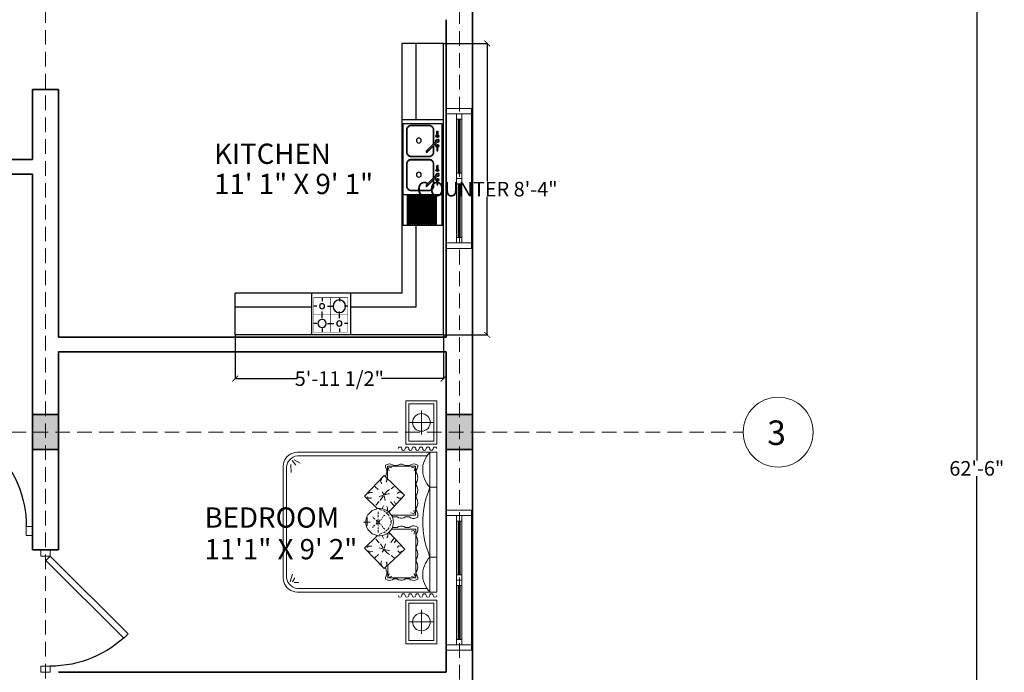
# Model space of a CAD drawing. Units: inches. Extents: x 782 to 2660, y -1008 to 166.
# Tile 6 of 12: x 1251 to 1589, y -400 to -176. Entities that reach past the tile are written whole.
import ezdxf

# ---------------------------------------------------------------- set-up
doc = ezdxf.new("R2010")
doc.units = ezdxf.units.IN
doc.header["$MEASUREMENT"] = 0
doc.linetypes.add('DASHED', pattern=[0.75, 0.5, -0.25])
for name, color, linetype, lineweight in [('A-ANNO-DIMS', 4, 'Continuous', 18), ('A-AREA-IDEN', 4, 'Continuous', 18), ('A-COLS', 7, 'Continuous', 35), ('A-Door', 150, 'Continuous', 18), ('A-FLOR-FIXT', 9, 'Continuous', 18), ('A-FURN', 8, 'Continuous', 13), ('A-Glaz', 4, 'Continuous', 18), ('A-GRID', 8, 'DASHED', 13), ('A-GRID-IDEN', 7, 'Continuous', 18), ('A-WALL', 7, 'Continuous', 35)]:
    doc.layers.add(name, color=color, linetype=linetype, lineweight=lineweight)
doc.layers.add('NET 01', color=8, linetype='Continuous')
doc.layers.add('TEFRIS', color=11, linetype='Continuous')
doc.styles.get("Standard").update_dxf_attribs({"font": 'arial.ttf'})
doc.dimstyles.get("Standard").update_dxf_attribs({"dimtxt": 5, "dimasz": 2, "dimexe": 0.18, "dimexo": 0.0625, "dimgap": 0.09, "dimtad": 0, "dimtih": 1, "dimtoh": 1, "dimdec": 0, "dimzin": 0, "dimdsep": 46, "dimlunit": 3, "dimtxsty": 'Standard', "dimblk": 'ARCHTICK', "dimcen": 0.09, "dimadec": 0, "dimazin": 0, "dimtfac": 1, "dimtdec": 0, "dimtofl": 0, "dimtmove": 0, "dimatfit": 3, "dimfxl": 1, "dimtolj": 1, "dimtzin": 0, "dimarcsym": 0})

# ---------------------------------------------------------------- blocks, each defined once
blk = doc.blocks.new('A$C592222DF')
at = {"layer": 'A-Door'}
for points in [[(-0.0354, -0.0354), (-0.6718, 0.601), (-0.6364, 0.6364), (0, 0)], [(-0.95, 0), (-0.95, -0.075), (-0.9, -0.075), (-0.9, 0)], [(0, 0), (0, -0.075), (0.05, -0.075), (0.05, 0)]]:
    blk.add_lwpolyline(points, close=True, dxfattribs=at)
at = {"layer": 'NET 01'}
blk.add_arc((0, 0), 0.9, 135, 180, dxfattribs=at)
blk = doc.blocks.new('d-bed-4')
at = {"color": 0, "linetype": 'ByBlock'}
for p, q in [((0.56, 0), (0, 0)), ((0, 0), (0, -0.4)), ((0.56, -0.4), (0.56, 0)), ((0.664, -1.8), (0.664, 0)), ((0.664, 0), (2.464, 0)), ((0.664, 0), (2.464, 0)), ((0.664, -1.8), (0.664, 0)), ((1.114, 0), (1.114, -0.09)), ((2.014, 0), (2.014, -0.09)), ((2.464, 0), (2.464, -1.8)), ((2.464, 0), (2.464, -1.8)), ((2.568, -0.4), (2.568, 0)), ((2.568, 0), (3.128, 0)), ((3.128, 0), (3.128, -0.4)), ((0.52, -0.04), (0.04, -0.04)), ((0.04, -0.04), (0.04, -0.36)), ((0.28, -0.046), (0.28, -0.354)), ((0.52, -0.36), (0.52, -0.04)), ((2.464, -0.09), (0.664, -0.09)), ((0.664, -0.09), (0.689, -0.112)), ((0.689, -0.112), (0.716, -0.131)), ((1.064, -0.131), (1.091, -0.112)), ((1.091, -0.112), (1.114, -0.09)), ((1.114, -0.09), (1.181, -0.115)), ((1.181, -0.115), (1.249, -0.137)), ((1.879, -0.137), (1.947, -0.115)), ((1.947, -0.115), (2.014, -0.09)), ((2.014, -0.09), (2.037, -0.112)), ((2.037, -0.112), (2.064, -0.131)), ((2.412, -0.131), (2.439, -0.112)), ((2.439, -0.112), (2.464, -0.09)), ((2.608, -0.36), (2.608, -0.04)), ((2.608, -0.04), (3.088, -0.04)), ((2.848, -0.046), (2.848, -0.354)), ((3.088, -0.04), (3.088, -0.36)), ((0.126, -0.2), (0.434, -0.2)), ((0.709, -1.795), (0.709, -0.128)), ((0.716, -0.131), (0.745, -0.148)), ((0.745, -0.148), (0.776, -0.162)), ((0.776, -0.162), (0.806, -0.173)), ((0.806, -0.173), (0.84, -0.18)), ((0.821, -0.268), (0.831, -0.248)), ((0.831, -0.248), (0.853, -0.248)), ((0.84, -0.18), (0.873, -0.184)), ((0.853, -0.248), (0.875, -0.256)), ((0.873, -0.184), (0.907, -0.184)), ((0.907, -0.184), (0.939, -0.18)), ((0.939, -0.18), (0.972, -0.173)), ((0.947, -0.256), (0.968, -0.25)), ((0.968, -0.25), (0.99, -0.248)), ((0.972, -0.173), (1.004, -0.162)), ((0.99, -0.248), (1.013, -0.25)), ((1.004, -0.162), (1.035, -0.148)), ((1.013, -0.25), (1.035, -0.256)), ((1.035, -0.148), (1.064, -0.131)), ((1.109, -0.256), (1.13, -0.25)), ((1.13, -0.25), (1.152, -0.248)), ((1.152, -0.248), (1.175, -0.25)), ((1.175, -0.25), (1.197, -0.256)), ((1.249, -0.137), (1.317, -0.155)), ((1.269, -0.256), (1.29, -0.25)), ((1.29, -0.25), (1.314, -0.248)), ((1.314, -0.248), (1.337, -0.25)), ((1.317, -0.155), (1.388, -0.169)), ((1.337, -0.25), (1.359, -0.256)), ((1.388, -0.169), (1.458, -0.178)), ((1.431, -0.256), (1.451, -0.248)), ((1.451, -0.248), (1.474, -0.248)), ((1.458, -0.178), (1.528, -0.182)), ((1.474, -0.248), (1.501, -0.248)), ((1.501, -0.248), (1.51, -0.268)), ((1.528, -0.182), (1.6, -0.182)), ((1.6, -0.182), (1.67, -0.178)), ((1.627, -0.248), (1.618, -0.268)), ((1.654, -0.248), (1.627, -0.248)), ((1.677, -0.248), (1.654, -0.248)), ((1.67, -0.178), (1.74, -0.169)), ((1.697, -0.256), (1.677, -0.248)), ((1.74, -0.169), (1.811, -0.155)), ((1.791, -0.25), (1.769, -0.256)), ((1.814, -0.248), (1.791, -0.25)), ((1.811, -0.155), (1.879, -0.137)), ((1.838, -0.25), (1.814, -0.248)), ((1.859, -0.256), (1.838, -0.25)), ((1.953, -0.25), (1.931, -0.256)), ((1.976, -0.248), (1.953, -0.25)), ((1.998, -0.25), (1.976, -0.248)), ((2.019, -0.256), (1.998, -0.25)), ((2.064, -0.131), (2.093, -0.148)), ((2.093, -0.148), (2.124, -0.162)), ((2.115, -0.25), (2.093, -0.256)), ((2.138, -0.248), (2.115, -0.25)), ((2.124, -0.162), (2.156, -0.173)), ((2.16, -0.25), (2.138, -0.248)), ((2.156, -0.173), (2.189, -0.18)), ((2.181, -0.256), (2.16, -0.25)), ((2.189, -0.18), (2.221, -0.184)), ((2.221, -0.184), (2.255, -0.184)), ((2.275, -0.248), (2.253, -0.256)), ((2.255, -0.184), (2.288, -0.18)), ((2.297, -0.248), (2.275, -0.248)), ((2.288, -0.18), (2.322, -0.173)), ((2.307, -0.268), (2.297, -0.248)), ((2.322, -0.173), (2.352, -0.162)), ((2.352, -0.162), (2.383, -0.148)), ((2.383, -0.148), (2.412, -0.131)), ((2.419, -0.128), (2.419, -1.795)), ((3.002, -0.2), (2.694, -0.2)), ((0.04, -0.36), (0.52, -0.36)), ((0.815, -0.292), (0.821, -0.268)), ((0.817, -0.315), (0.815, -0.292)), ((0.824, -0.337), (0.817, -0.315)), ((0.835, -0.356), (0.824, -0.337)), ((0.835, -0.405), (0.835, -0.356)), ((0.844, -0.635), (0.844, -0.275)), ((0.844, -0.275), (1.472, -0.275)), ((0.857, -0.293), (0.866, -0.329)), ((0.862, -0.281), (0.902, -0.293)), ((0.875, -0.256), (0.894, -0.266)), ((0.894, -0.266), (0.925, -0.266)), ((0.925, -0.266), (0.947, -0.256)), ((1.035, -0.256), (1.056, -0.266)), ((1.056, -0.266), (1.087, -0.266)), ((1.087, -0.266), (1.109, -0.256)), ((1.197, -0.256), (1.217, -0.266)), ((1.217, -0.266), (1.249, -0.266)), ((1.249, -0.266), (1.269, -0.256)), ((1.359, -0.256), (1.379, -0.266)), ((1.379, -0.266), (1.411, -0.266)), ((1.451, -0.284), (1.409, -0.299)), ((1.411, -0.266), (1.431, -0.256)), ((1.454, -0.299), (1.445, -0.335)), ((1.472, -0.275), (1.472, -0.581)), ((1.508, -0.337), (1.496, -0.356)), ((1.496, -0.356), (1.496, -0.405)), ((1.515, -0.315), (1.508, -0.337)), ((1.51, -0.268), (1.515, -0.292)), ((1.515, -0.292), (1.515, -0.315)), ((1.618, -0.268), (1.613, -0.292)), ((1.613, -0.292), (1.613, -0.315)), ((1.613, -0.315), (1.62, -0.337)), ((1.62, -0.337), (1.632, -0.356)), ((1.632, -0.356), (1.632, -0.405)), ((2.282, -0.274), (1.654, -0.274)), ((1.654, -0.274), (1.654, -0.58)), ((1.672, -0.297), (1.681, -0.333)), ((1.676, -0.283), (1.717, -0.297)), ((1.717, -0.266), (1.697, -0.256)), ((1.749, -0.266), (1.717, -0.266)), ((1.769, -0.256), (1.749, -0.266)), ((1.879, -0.266), (1.859, -0.256)), ((1.911, -0.266), (1.879, -0.266)), ((1.931, -0.256), (1.911, -0.266)), ((2.041, -0.266), (2.019, -0.256)), ((2.072, -0.266), (2.041, -0.266)), ((2.093, -0.256), (2.072, -0.266)), ((2.203, -0.266), (2.181, -0.256)), ((2.234, -0.266), (2.203, -0.266)), ((2.264, -0.279), (2.225, -0.292)), ((2.253, -0.256), (2.234, -0.266)), ((2.27, -0.292), (2.261, -0.328)), ((2.282, -0.634), (2.282, -0.274)), ((2.293, -0.356), (2.304, -0.337)), ((2.293, -0.405), (2.293, -0.356)), ((2.304, -0.337), (2.311, -0.315)), ((2.313, -0.292), (2.307, -0.268)), ((2.311, -0.315), (2.313, -0.292)), ((3.088, -0.36), (2.608, -0.36)), ((0, -0.4), (0.56, -0.4)), ((0.819, -0.448), (0.824, -0.425)), ((0.819, -0.47), (0.819, -0.448)), ((0.824, -0.493), (0.819, -0.47)), ((0.824, -0.425), (0.835, -0.405)), ((0.835, -0.513), (0.824, -0.493)), ((0.965, -0.68), (1.217, -0.416)), ((1.19, -0.452), (1.172, -0.482)), ((1.172, -0.482), (1.193, -0.506)), ((1.217, -0.416), (1.433, -0.621)), ((1.256, -0.491), (1.238, -0.515)), ((1.253, -0.446), (1.256, -0.491)), ((1.496, -0.405), (1.508, -0.425)), ((1.508, -0.493), (1.496, -0.513)), ((1.508, -0.425), (1.514, -0.448)), ((1.514, -0.47), (1.508, -0.493)), ((1.514, -0.448), (1.514, -0.47)), ((1.62, -0.425), (1.614, -0.448)), ((1.614, -0.448), (1.614, -0.47)), ((1.614, -0.47), (1.62, -0.493)), ((1.632, -0.405), (1.62, -0.425)), ((1.62, -0.493), (1.632, -0.513)), ((1.91, -0.414), (1.694, -0.619)), ((1.874, -0.445), (1.87, -0.49)), ((1.87, -0.49), (1.888, -0.513)), ((2.162, -0.679), (1.91, -0.414)), ((1.955, -0.481), (1.933, -0.504)), ((1.937, -0.45), (1.955, -0.481)), ((2.304, -0.425), (2.293, -0.405)), ((2.293, -0.513), (2.304, -0.493)), ((2.309, -0.448), (2.304, -0.425)), ((2.304, -0.493), (2.309, -0.47)), ((2.309, -0.47), (2.309, -0.448)), ((3.128, -0.4), (2.568, -0.4)), ((0.815, -0.617), (0.817, -0.594)), ((0.821, -0.641), (0.815, -0.617)), ((0.817, -0.594), (0.824, -0.572)), ((0.824, -0.572), (0.835, -0.553)), ((0.835, -0.553), (0.835, -0.513)), ((0.857, -0.617), (0.866, -0.581)), ((0.862, -0.63), (0.902, -0.617)), ((1.105, -0.551), (1.136, -0.59)), ((1.163, -0.639), (1.145, -0.612)), ((1.199, -0.626), (1.199, -0.612)), ((1.211, -0.675), (1.199, -0.626)), ((1.328, -0.533), (1.298, -0.551)), ((1.355, -0.551), (1.301, -0.596)), ((1.409, -0.612), (1.433, -0.621)), ((1.411, -0.652), (1.425, -0.63)), ((1.425, -0.63), (1.443, -0.61)), ((1.465, -0.626), (1.438, -0.659)), ((1.443, -0.61), (1.463, -0.592)), ((1.463, -0.592), (1.487, -0.578)), ((1.465, -0.626), (1.483, -0.617)), ((1.487, -0.578), (1.512, -0.567)), ((1.496, -0.513), (1.496, -0.567)), ((1.528, -0.596), (1.501, -0.608)), ((1.512, -0.567), (1.537, -0.562)), ((1.537, -0.562), (1.564, -0.558)), ((1.537, -0.59), (1.562, -0.59)), ((1.58, -0.59), (1.555, -0.59)), ((1.559, -0.587), (1.559, -0.599)), ((1.559, -0.587), (1.559, -0.599)), ((1.564, -0.558), (1.591, -0.562)), ((1.589, -0.596), (1.616, -0.608)), ((1.591, -0.562), (1.616, -0.567)), ((1.616, -0.567), (1.641, -0.578)), ((1.632, -0.513), (1.632, -0.567)), ((1.652, -0.626), (1.634, -0.617)), ((1.641, -0.578), (1.665, -0.592)), ((1.665, -0.592), (1.685, -0.61)), ((1.685, -0.61), (1.703, -0.63)), ((1.717, -0.61), (1.694, -0.619)), ((1.703, -0.63), (1.717, -0.652)), ((1.771, -0.549), (1.825, -0.594)), ((1.798, -0.531), (1.829, -0.549)), ((1.915, -0.673), (1.928, -0.625)), ((1.928, -0.625), (1.928, -0.61)), ((1.964, -0.637), (1.982, -0.61)), ((2.021, -0.549), (1.991, -0.589)), ((2.264, -0.628), (2.225, -0.616)), ((2.27, -0.616), (2.261, -0.58)), ((2.293, -0.553), (2.293, -0.513)), ((2.304, -0.572), (2.293, -0.553)), ((2.311, -0.594), (2.304, -0.572)), ((2.307, -0.641), (2.313, -0.617)), ((2.313, -0.617), (2.311, -0.594)), ((0.831, -0.661), (0.821, -0.641)), ((0.853, -0.661), (0.831, -0.661)), ((1.01, -0.635), (0.844, -0.635)), ((0.875, -0.653), (0.853, -0.661)), ((0.894, -0.643), (0.875, -0.653)), ((0.907, -0.644), (0.893, -0.644)), ((0.925, -0.643), (0.894, -0.643)), ((0.916, -0.644), (0.907, -0.644)), ((0.925, -0.644), (0.916, -0.644)), ((0.947, -0.653), (0.925, -0.643)), ((0.968, -0.659), (0.947, -0.653)), ((1.229, -0.932), (0.965, -0.68)), ((0.983, -0.661), (0.968, -0.659)), ((1.006, -0.644), (1.024, -0.644)), ((1.006, -0.711), (1.037, -0.725)), ((1.024, -0.644), (1.042, -0.653)), ((1.042, -0.653), (1.028, -0.644)), ((1.028, -0.644), (1.051, -0.648)), ((1.037, -0.725), (1.055, -0.716)), ((1.055, -0.716), (1.064, -0.711)), ((1.105, -0.801), (1.145, -0.756)), ((1.202, -0.675), (1.163, -0.639)), ((1.175, -0.707), (1.208, -0.684)), ((1.22, -0.707), (1.211, -0.675)), ((1.226, -0.68), (1.283, -0.666)), ((1.226, -0.711), (1.235, -0.743)), ((1.229, -0.693), (1.283, -0.729)), ((1.343, -0.788), (1.298, -0.743)), ((1.379, -0.702), (1.352, -0.689)), ((1.382, -0.635), (1.361, -0.644)), ((1.379, -0.702), (1.391, -0.702)), ((1.415, -0.635), (1.382, -0.635)), ((1.389, -0.729), (1.393, -0.702)), ((1.389, -0.756), (1.389, -0.729)), ((1.395, -0.781), (1.389, -0.756)), ((1.393, -0.702), (1.4, -0.677)), ((1.397, -0.743), (1.411, -0.711)), ((1.4, -0.677), (1.411, -0.652)), ((1.415, -0.635), (1.418, -0.639)), ((1.42, -0.677), (1.415, -0.695)), ((1.42, -0.677), (1.429, -0.668)), ((1.46, -0.756), (1.429, -0.756)), ((1.438, -0.635), (1.442, -0.641)), ((1.487, -0.686), (1.474, -0.671)), ((1.496, -0.756), (1.474, -0.756)), ((1.514, -0.707), (1.496, -0.695)), ((1.514, -0.756), (1.51, -0.756)), ((1.532, -0.72), (1.523, -0.72)), ((1.55, -0.765), (1.523, -0.756)), ((1.559, -0.747), (1.537, -0.729)), ((1.55, -0.756), (1.55, -0.747)), ((1.55, -0.747), (1.559, -0.747)), ((1.55, -0.765), (1.55, -0.756)), ((1.559, -0.747), (1.562, -0.745)), ((1.568, -0.747), (1.562, -0.745)), ((1.568, -0.747), (1.589, -0.729)), ((1.577, -0.747), (1.568, -0.747)), ((1.577, -0.756), (1.577, -0.747)), ((1.577, -0.765), (1.577, -0.756)), ((1.577, -0.765), (1.604, -0.756)), ((1.595, -0.72), (1.604, -0.72)), ((1.613, -0.707), (1.631, -0.695)), ((1.613, -0.756), (1.616, -0.756)), ((1.631, -0.756), (1.652, -0.756)), ((1.64, -0.686), (1.652, -0.671)), ((1.659, -0.635), (1.681, -0.657)), ((1.667, -0.756), (1.697, -0.756)), ((1.697, -0.677), (1.688, -0.668)), ((1.697, -0.677), (1.703, -0.695)), ((1.721, -0.743), (1.706, -0.711)), ((1.712, -0.634), (1.708, -0.637)), ((1.712, -0.634), (1.744, -0.634)), ((1.717, -0.652), (1.728, -0.677)), ((1.728, -0.677), (1.735, -0.702)), ((1.739, -0.756), (1.733, -0.781)), ((1.748, -0.7), (1.735, -0.7)), ((1.735, -0.702), (1.739, -0.729)), ((1.739, -0.729), (1.739, -0.756)), ((1.744, -0.634), (1.766, -0.643)), ((1.748, -0.7), (1.775, -0.688)), ((1.784, -0.787), (1.829, -0.742)), ((1.901, -0.679), (1.843, -0.664)), ((1.897, -0.691), (1.843, -0.727)), ((1.901, -0.709), (1.892, -0.742)), ((1.897, -0.931), (2.162, -0.679)), ((1.906, -0.706), (1.915, -0.673)), ((1.951, -0.706), (1.919, -0.682)), ((1.924, -0.673), (1.964, -0.637)), ((2.021, -0.799), (1.982, -0.754)), ((2.072, -0.715), (2.063, -0.709)), ((2.09, -0.724), (2.072, -0.715)), ((2.099, -0.643), (2.075, -0.646)), ((2.102, -0.643), (2.084, -0.652)), ((2.084, -0.652), (2.099, -0.643)), ((2.12, -0.709), (2.09, -0.724)), ((2.12, -0.643), (2.102, -0.643)), ((2.117, -0.634), (2.282, -0.634)), ((2.145, -0.661), (2.16, -0.659)), ((2.16, -0.659), (2.181, -0.653)), ((2.181, -0.653), (2.203, -0.643)), ((2.201, -0.643), (2.21, -0.643)), ((2.203, -0.643), (2.234, -0.643)), ((2.21, -0.643), (2.219, -0.643)), ((2.219, -0.643), (2.234, -0.643)), ((2.234, -0.643), (2.253, -0.653)), ((2.253, -0.653), (2.275, -0.661)), ((2.275, -0.661), (2.297, -0.661)), ((2.297, -0.661), (2.307, -0.641)), ((1.181, -0.851), (1.184, -0.828)), ((1.181, -0.869), (1.181, -0.851)), ((1.193, -0.891), (1.181, -0.869)), ((1.229, -0.932), (1.388, -0.77)), ((1.238, -0.9), (1.253, -0.882)), ((1.253, -0.846), (1.247, -0.846)), ((1.253, -0.882), (1.253, -0.846)), ((1.404, -0.808), (1.395, -0.781)), ((1.415, -0.832), (1.404, -0.808)), ((1.431, -0.853), (1.415, -0.832)), ((1.451, -0.873), (1.431, -0.853)), ((1.47, -0.889), (1.451, -0.873)), ((1.501, -0.819), (1.496, -0.828)), ((1.523, -0.801), (1.51, -0.815)), ((1.532, -0.792), (1.532, -0.792)), ((1.559, -0.77), (1.537, -0.783)), ((1.559, -0.77), (1.55, -0.765)), ((1.559, -0.77), (1.562, -0.77)), ((1.568, -0.77), (1.562, -0.77)), ((1.564, -0.945), (1.564, -0.86)), ((1.568, -0.77), (1.577, -0.765)), ((1.568, -0.77), (1.589, -0.783)), ((1.595, -0.792), (1.595, -0.792)), ((1.604, -0.801), (1.616, -0.815)), ((1.625, -0.819), (1.631, -0.828)), ((1.677, -0.873), (1.658, -0.889)), ((1.697, -0.853), (1.677, -0.873)), ((1.713, -0.832), (1.697, -0.853)), ((1.724, -0.808), (1.713, -0.832)), ((1.733, -0.781), (1.724, -0.808)), ((1.897, -0.931), (1.739, -0.769)), ((1.874, -0.88), (1.874, -0.844)), ((1.874, -0.844), (1.879, -0.844)), ((1.888, -0.898), (1.874, -0.88)), ((1.933, -0.889), (1.946, -0.868)), ((1.946, -0.85), (1.942, -0.826)), ((1.946, -0.868), (1.946, -0.85)), ((1.496, -0.902), (1.47, -0.889)), ((1.521, -0.911), (1.496, -0.902)), ((1.609, -0.896), (1.503, -0.896)), ((1.546, -0.916), (1.521, -0.911)), ((1.564, -0.916), (1.546, -0.916)), ((1.582, -0.916), (1.564, -0.916)), ((1.607, -0.911), (1.582, -0.916)), ((1.632, -0.902), (1.607, -0.911)), ((1.658, -0.889), (1.632, -0.902)), ((0.763, -1.836), (0.803, -1.76)), ((0.668, -1.827), (0.664, -1.8)), ((0.668, -1.827), (0.664, -1.8)), ((0.675, -1.854), (0.668, -1.827)), ((0.675, -1.854), (0.668, -1.827)), ((0.686, -1.881), (0.675, -1.854)), ((0.686, -1.881), (0.675, -1.854)), ((0.7, -1.904), (0.686, -1.881)), ((0.7, -1.904), (0.686, -1.881)), ((0.716, -1.825), (0.709, -1.795)), ((0.727, -1.852), (0.716, -1.825)), ((0.745, -1.877), (0.727, -1.852)), ((0.767, -1.899), (0.745, -1.877)), ((0.792, -1.917), (0.767, -1.899)), ((0.772, -1.863), (0.83, -1.818)), ((0.821, -1.881), (0.925, -1.876)), ((2.333, -1.89), (2.234, -1.858)), ((2.333, -1.858), (2.282, -1.827)), ((2.361, -1.899), (2.336, -1.917)), ((2.342, -1.836), (2.342, -1.778)), ((2.383, -1.877), (2.361, -1.899)), ((2.401, -1.852), (2.383, -1.877)), ((2.412, -1.825), (2.401, -1.852)), ((2.419, -1.795), (2.412, -1.825)), ((2.442, -1.881), (2.428, -1.904)), ((2.442, -1.881), (2.428, -1.904)), ((2.453, -1.854), (2.442, -1.881)), ((2.453, -1.854), (2.442, -1.881)), ((2.46, -1.827), (2.453, -1.854)), ((2.46, -1.827), (2.453, -1.854)), ((2.464, -1.8), (2.46, -1.827)), ((2.464, -1.8), (2.46, -1.827)), ((0.718, -1.926), (0.7, -1.904)), ((0.718, -1.926), (0.7, -1.904)), ((0.74, -1.944), (0.718, -1.926)), ((0.74, -1.944), (0.718, -1.926)), ((0.763, -1.958), (0.74, -1.944)), ((0.763, -1.958), (0.74, -1.944)), ((0.79, -1.969), (0.763, -1.958)), ((0.79, -1.969), (0.763, -1.958)), ((0.817, -1.976), (0.79, -1.969)), ((0.817, -1.976), (0.79, -1.969)), ((0.819, -1.928), (0.792, -1.917)), ((0.844, -1.98), (0.817, -1.976)), ((0.844, -1.98), (0.817, -1.976)), ((0.849, -1.935), (0.819, -1.928)), ((2.284, -1.98), (0.844, -1.98)), ((2.284, -1.98), (0.844, -1.98)), ((2.279, -1.935), (0.849, -1.935)), ((2.309, -1.928), (2.279, -1.935)), ((2.311, -1.976), (2.284, -1.98)), ((2.311, -1.976), (2.284, -1.98)), ((2.336, -1.917), (2.309, -1.928)), ((2.338, -1.969), (2.311, -1.976)), ((2.338, -1.969), (2.311, -1.976)), ((2.365, -1.958), (2.338, -1.969)), ((2.365, -1.958), (2.338, -1.969)), ((2.388, -1.944), (2.365, -1.958)), ((2.388, -1.944), (2.365, -1.958)), ((2.41, -1.926), (2.388, -1.944)), ((2.41, -1.926), (2.388, -1.944)), ((2.428, -1.904), (2.41, -1.926)), ((2.428, -1.904), (2.41, -1.926))]:
    blk.add_line(p, q, dxfattribs=at)
for centre in [(0.28, -0.2), (2.848, -0.2)]:
    blk.add_ellipse(centre, major_axis=(-0.0806, 0.0806), ratio=1, dxfattribs=at)
for centre, major_axis, start_param, end_param in [((0.617, -0.026), (-0.0159, 0.0159), 5.497787, 8.63938), ((0.617, -0.116), (-0.0159, 0.0159), 5.497787, 8.63938), ((0.617, -0.071), (-0.0159, 0.0159), 2.356194, 5.497787), ((2.507, -0.071), (0.0159, 0.0159), 0.785398, 3.926991), ((2.507, -0.026), (0.0159, 0.0159), 3.926991, 7.068583), ((2.507, -0.116), (0.0159, 0.0159), 3.926991, 7.068583), ((0.617, -0.206), (-0.0159, 0.0159), 5.497787, 8.63938), ((0.617, -0.161), (-0.0159, 0.0159), 2.356194, 5.497787), ((0.617, -0.161), (-0.0159, 0.0159), 2.356194, 5.497787), ((0.617, -0.251), (-0.0159, 0.0159), 2.356194, 5.497787), ((2.507, -0.161), (0.0159, 0.0159), 0.785398, 3.926991), ((2.507, -0.161), (0.0159, 0.0159), 0.785398, 3.926991), ((2.507, -0.251), (0.0159, 0.0159), 0.785398, 3.926991), ((2.507, -0.206), (0.0159, 0.0159), 3.926991, 7.068583), ((0.617, -0.296), (-0.0159, 0.0159), 5.497787, 8.63938), ((0.617, -0.386), (-0.0159, 0.0159), 5.497787, 8.63938), ((0.617, -0.341), (-0.0159, 0.0159), 2.356194, 5.497787), ((2.507, -0.341), (0.0159, 0.0159), 0.785398, 3.926991), ((2.507, -0.296), (0.0159, 0.0159), 3.926991, 7.068583), ((2.507, -0.386), (0.0159, 0.0159), 3.926991, 7.068583), ((0.617, -0.476), (-0.0159, 0.0159), 5.497787, 8.63938), ((0.617, -0.431), (-0.0159, 0.0159), 2.356194, 5.497787), ((2.507, -0.431), (0.0159, 0.0159), 0.785398, 3.926991), ((2.507, -0.476), (0.0159, 0.0159), 3.926991, 7.068583)]:
    blk.add_ellipse(centre, major_axis=major_axis, ratio=1, start_param=start_param, end_param=end_param, dxfattribs=at)
blk = doc.blocks.new('A$C2CE61BFE')
at = {"layer": 'TEFRIS'}
for p, q in [((12.7, 50), (12.7, 45)), ((37.6, 50), (37.6, 45)), ((5.3, 37.6), (0.3, 37.6)), ((12.7, 20.5), (12.7, 29.8)), ((20.5, 37.6), (29.8, 37.6)), ((37.6, 20.5), (37.6, 29.8)), ((50, 37.6), (45, 37.6)), ((5.3, 12.7), (0.3, 12.7)), ((12.7, 5.3), (12.7, 0.3)), ((20.5, 12.7), (29.8, 12.7)), ((37.6, 5.3), (37.6, 0.3)), ((50, 12.7), (45, 12.7))]:
    blk.add_line(p, q, dxfattribs=at)
at = {"layer": 'TEFRIS', "const_width": 0.617}
blk.add_lwpolyline([(50, 50), (0.3, 50), (0.3, 0.3), (50, 0.3)], close=True, dxfattribs=at)
at = {"layer": 'TEFRIS', "const_width": 0.514}
for points in [[(25.1, 50), (25.1, 0.3)], [(50, 25.1), (0.3, 25.1)]]:
    blk.add_lwpolyline(points, dxfattribs=at)
at = {"layer": 'TEFRIS'}
for centre, radius in [((37.6, 37.6), 9.04), ((12.7, 37.6), 3.83), ((12.7, 12.7), 5.97), ((37.6, 12.7), 3.62)]:
    blk.add_circle(centre, radius, dxfattribs=at)
blk = doc.blocks.new('A$C59F64124')
at = {"layer": 'TEFRIS'}
for p, q in [((0, 0), (0, 60)), ((146.8, 57.7), (0, 57.7)), ((44.5, 2.1), (44.5, 57.7)), ((146.8, 2.1), (146.8, 57.7)), ((0, 2.1), (146.8, 2.1))]:
    blk.add_line(p, q, dxfattribs=at)
for points in [[(2.2, 49.9), (42.3, 49.9, -1), (42.3, 47.7), (2.2, 47.7, -1), (2.2, 49.9)], [(2.2, 46.6), (42.3, 46.6, -1), (42.3, 44.4), (2.2, 44.4, -1), (2.2, 46.6)], [(2.2, 43.3), (42.3, 43.3, -1), (42.3, 41), (2.2, 41, -1), (2.2, 43.3)], [(65.3, 45.7), (56.2, 45.7, 0.414214), (49.5, 39)], [(49.5, 39), (49.5, 13.7, 0.414214), (56.2, 7), (88.6, 7, 0.414214), (95.3, 13.7), (95.3, 39, 0.414214), (88.6, 45.7), (68.3, 45.7, 0.414214)], [(64.7, 45.1), (56.2, 45.1, 0.414214), (50.2, 39)], [(50.2, 39), (50.2, 13.7, 0.414214), (56.2, 7.7), (88.6, 7.7, 0.414214), (94.6, 13.7), (94.6, 39, 0.414214), (88.6, 45.1), (67.7, 45.1, 0.414214)], [(114.5, 45.7), (105.3, 45.7, 0.414214), (98.7, 39)], [(98.7, 39), (98.7, 13.7, 0.414214), (105.3, 7), (137.8, 7, 0.414214), (144.4, 13.7), (144.4, 39, 0.414214), (137.8, 45.7), (117.5, 45.7, 0.330435)], [(113.8, 45.1), (105.3, 45.1, 0.414214), (99.3, 39)], [(99.3, 39), (99.3, 13.7, 0.414214), (105.3, 7.7), (137.8, 7.7, 0.414214), (143.8, 13.7), (143.8, 39, 0.414214), (137.8, 45.1), (116.8, 45.1, 0.333106)], [(2.2, 39.9), (42.3, 39.9, -1), (42.3, 37.7), (2.2, 37.7, -1), (2.2, 39.9)], [(2.2, 36.6), (42.3, 36.6, -1), (42.3, 34.4), (2.2, 34.4, -1), (2.2, 36.6)], [(2.2, 33.2), (42.3, 33.2, -1), (42.3, 31), (2.2, 31, -1), (2.2, 33.2)], [(2.2, 29.9), (42.3, 29.9, -1), (42.3, 27.7), (2.2, 27.7, -1), (2.2, 29.9)], [(2.2, 26.6), (42.3, 26.6, -1), (42.3, 24.3), (2.2, 24.3, -1), (2.2, 26.6)], [(2.2, 23.2), (42.3, 23.2, -1), (42.3, 21), (2.2, 21, -1), (2.2, 23.2)], [(2.2, 19.9), (42.3, 19.9, -1), (42.3, 17.7), (2.2, 17.7, -1), (2.2, 19.9)], [(2.2, 16.5), (42.3, 16.5, -1), (42.3, 14.3), (2.2, 14.3, -1), (2.2, 16.5)], [(2.2, 13.2), (42.3, 13.2, -1), (42.3, 11), (2.2, 11, -1), (2.2, 13.2)], [(2.2, 9.9), (42.3, 9.9, -1), (42.3, 7.6), (2.2, 7.6, -1), (2.2, 9.9)]]:
    blk.add_lwpolyline(points, format="xyb", dxfattribs=at)
for points in [[(56.4, 36.7), (73.1, 53.5, -1), (74.6, 52), (57.9, 35.2, -1)], [(58.9, 52), (66.5, 52, -0.563183), (66.5, 50.5), (58.9, 50.5, -1)], [(85.8, 52), (78.2, 52, 0.563183), (78.2, 50.5), (85.8, 50.5, 1)], [(105.5, 36.7), (122.3, 53.5, -1), (123.8, 52), (107, 35.2, -1)], [(108, 52), (115.7, 52, -0.563183), (115.7, 50.5), (108, 50.5, -1)], [(135, 52), (127.4, 52, 0.563183), (127.4, 50.5), (135, 50.5, 1)]]:
    blk.add_lwpolyline(points, format="xyb", close=True, dxfattribs=at)
for centre, radius in [((58.2, 37.1), 0.707), ((107.4, 37.1), 0.707), ((72.9, 24.5), 3.54), ((122.1, 24.5), 3.54)]:
    blk.add_circle(centre, radius, dxfattribs=at)
for centre, start, end in [((65.2, 51.2), 199.4712, 160.5288), ((72.4, 51.2), 75, 195), ((72.4, 51.2), 255, 15), ((79.5, 51.2), 19.4712, 340.5288), ((114.4, 51.2), 199.4712, 160.5288), ((121.5, 51.2), 75, 195), ((121.5, 51.2), 255, 15), ((128.6, 51.2), 19.4712, 340.5288)]:
    blk.add_arc(centre, 2.12, start, end, dxfattribs=at)
blk = doc.blocks.new('A$C344845E7')
at = {"layer": 'TEFRIS'}
for p, q in [((-0.6, 4.2), (-0.6, 0.6)), ((0, 4.2), (-0.6, 4.2)), ((-0.4, 4.2), (-0.4, 3.1)), ((0, 0), (0, 4.2)), ((0, 3.1), (-0.6, 3.1)), ((-0.4, 1.579), (-0.4, 0.4)), ((-2.999, 0), (-2.999, 0.6)), ((-0.6, 0.6), (-2.999, 0.6)), ((-1.9, 0.6), (-1.9, 0)), ((-1.34, 0.6), (-1.34, 0)), ((-1.9, 0.4), (-2.999, 0.4)), ((-0.4, 0.4), (-1.34, 0.4)), ((0, 0), (-2.999, 0))]:
    blk.add_line(p, q, dxfattribs=at)
at = {"layer": 'TEFRIS', "xscale": -0.01, "yscale": 0.01, "zscale": 0.01, "rotation": 270}
for name, p in [('A$C59F64124', (-0.6, 1.579)), ('A$C2CE61BFE', (-1.876, 0.037))]:
    blk.add_blockref(name, p, dxfattribs=at)
blk = doc.blocks.new('WIN-48-FRAME-B')
for p, q in [((8.69, 48), (0, 48)), ((0, 48), (0, 46.15)), ((8.69, 48), (0, 48)), ((8.69, 0), (8.69, 48)), ((8.69, 46.15), (8.69, 48)), ((0, 46.15), (8.69, 46.15)), ((0, 46.15), (8.69, 46.15)), ((0, 1.85), (0, 46.15)), ((3.5, 46.15), (3.5, 1.85)), ((3.5, 44.31), (5.35, 44.31)), ((4.05, 44.31), (4.05, 25.85)), ((4.42, 44.31), (4.42, 25.85)), ((4.79, 44.31), (4.79, 25.85)), ((5.35, 46.15), (5.35, 1.85)), ((5.35, 25.85), (3.5, 25.85)), ((5.35, 24), (3.5, 24)), ((5.35, 22.15), (3.5, 22.15)), ((4.05, 3.69), (4.05, 22.15)), ((4.42, 3.69), (4.42, 22.15)), ((4.79, 3.69), (4.79, 22.15)), ((3.5, 3.69), (5.35, 3.69)), ((0, 1.85), (8.69, 1.85)), ((0, 0), (0, 1.85)), ((0, 1.85), (8.69, 1.85)), ((0, 1.85), (8.69, 1.85)), ((8.69, 0), (0, 0)), ((0, 0), (8.69, 0)), ((8.69, 1.85), (8.69, 0))]:
    blk.add_line(p, q)
blk = doc.blocks.new('COL-9X12')
h = blk.add_hatch(color=256)
h.dxf.hatch_style = 1
h.paths.add_polyline_path([(9, 12), (0, 12), (0, 0), (9, 0)])
blk.add_lwpolyline([(0, 12), (9, 12), (9, 0), (0, 0)], close=True)
blk = doc.blocks.new('_ArchTick')
at = {"color": 0, "linetype": 'ByBlock', "const_width": 0.15}
blk.add_lwpolyline([(-0.5, -0.5), (0.5, 0.5)], dxfattribs=at)
blk = doc.blocks.new('*D38')
at = {"layer": 'A-ANNO-DIMS', "color": 0, "lineweight": -2, "transparency": 16777216}
for p, q in [((1397.68, -416.93), (1397.68, -409.61)), ((1397.68, -409.79), (1406.38, -409.79)), ((1406.38, -416.93), (1406.38, -409.61)), ((1406.38, -409.79), (1408.38, -409.79))]:
    blk.add_line(p, q, dxfattribs=at)
at = {"layer": 'Defpoints', "color": 0, "transparency": 16777216}
for p in [(1406.38, -409.79), (1397.68, -416.99), (1406.38, -416.99)]:
    blk.add_point(p, dxfattribs=at)
at = {"layer": 'A-ANNO-DIMS', "color": 0, "lineweight": -2, "transparency": 16777216, "xscale": 2, "yscale": 2, "zscale": 2, "rotation": 180}
blk.add_blockref('_ArchTick', (1397.68, -409.79), dxfattribs=at)
at = {"layer": 'A-ANNO-DIMS', "color": 0, "lineweight": -2, "transparency": 16777216, "xscale": 2, "yscale": 2, "zscale": 2}
blk.add_blockref('_ArchTick', (1406.38, -409.79), dxfattribs=at)
at = {"layer": 'A-ANNO-DIMS', "color": 0, "transparency": 16777216, "insert": (1429.53, -409.79), "char_height": 5, "attachment_point": 5}
blk.add_mtext('\\A1;0\'-8 1/2" TYP.', dxfattribs=at)
blk = doc.blocks.new('*D43')
at = {"layer": 'A-ANNO-DIMS', "color": 0, "lineweight": -2, "transparency": 16777216}
for p, q in [((1396.78, -184.14), (1411.9, -184.14)), ((1411.72, -184.14), (1411.72, -231.48)), ((1411.72, -284.18), (1411.72, -236.84)), ((1396.78, -284.18), (1411.9, -284.18))]:
    blk.add_line(p, q, dxfattribs=at)
at = {"layer": 'Defpoints', "color": 0, "transparency": 16777216}
for p in [(1396.72, -184.14), (1411.72, -184.14), (1396.72, -284.18)]:
    blk.add_point(p, dxfattribs=at)
at = {"layer": 'A-ANNO-DIMS', "color": 0, "lineweight": -2, "transparency": 16777216, "xscale": 2, "yscale": 2, "zscale": 2}
for p, rotation in [((1411.72, -184.14), 90), ((1411.72, -284.18), 270)]:
    blk.add_blockref('_ArchTick', p, dxfattribs=dict(at, rotation=rotation))
at = {"layer": 'A-ANNO-DIMS', "color": 0, "transparency": 16777216, "insert": (1411.72, -234.16), "char_height": 5, "attachment_point": 5}
blk.add_mtext('\\A1;COUNTER 8\'-4"', dxfattribs=at)
blk = doc.blocks.new('*D44')
at = {"layer": 'A-ANNO-DIMS', "color": 0, "lineweight": -2, "transparency": 16777216}
for p, q in [((1325.28, -284.24), (1325.28, -299.36)), ((1396.72, -284.24), (1396.72, -299.36)), ((1325.28, -299.18), (1346.5, -299.18)), ((1396.72, -299.18), (1375.5, -299.18))]:
    blk.add_line(p, q, dxfattribs=at)
at = {"layer": 'Defpoints', "color": 0, "transparency": 16777216}
for p in [(1325.28, -284.18), (1396.72, -284.18), (1396.72, -299.18)]:
    blk.add_point(p, dxfattribs=at)
at = {"layer": 'A-ANNO-DIMS', "color": 0, "lineweight": -2, "transparency": 16777216, "xscale": 2, "yscale": 2, "zscale": 2, "rotation": 180}
blk.add_blockref('_ArchTick', (1325.28, -299.18), dxfattribs=at)
at = {"layer": 'A-ANNO-DIMS', "color": 0, "lineweight": -2, "transparency": 16777216, "xscale": 2, "yscale": 2, "zscale": 2}
blk.add_blockref('_ArchTick', (1396.72, -299.18), dxfattribs=at)
at = {"layer": 'A-ANNO-DIMS', "color": 0, "transparency": 16777216, "insert": (1361, -299.18), "char_height": 5, "attachment_point": 5}
blk.add_mtext('\\A1;5\'-11 1/2"', dxfattribs=at)
blk = doc.blocks.new('*D51')
at = {"layer": 'A-ANNO-DIMS', "color": 0, "lineweight": -2, "transparency": 16777216}
for p, q in [((1406.75, 45.01), (1579.89, 45.01)), ((1579.71, 45.01), (1579.71, -327.35)), ((1579.71, -704.99), (1579.71, -332.64)), ((1406.75, -704.99), (1579.89, -704.99))]:
    blk.add_line(p, q, dxfattribs=at)
at = {"layer": 'Defpoints', "color": 0, "transparency": 16777216}
for p in [(1406.68, 45.01), (1579.71, 45.01), (1406.68, -704.99)]:
    blk.add_point(p, dxfattribs=at)
at = {"layer": 'A-ANNO-DIMS', "color": 0, "lineweight": -2, "transparency": 16777216, "xscale": 2, "yscale": 2, "zscale": 2}
for p, rotation in [((1579.71, 45.01), 90), ((1579.71, -704.99), 270)]:
    blk.add_blockref('_ArchTick', p, dxfattribs=dict(at, rotation=rotation))
at = {"layer": 'A-ANNO-DIMS', "color": 0, "transparency": 16777216, "insert": (1579.71, -329.99), "char_height": 5, "attachment_point": 5}
blk.add_mtext('\\A1;62\'-6"', dxfattribs=at)

msp = doc.modelspace()

# ---------------------------------------------------------------- linework, layer by layer
at = {"layer": 'A-GRID', "ltscale": 10}
for p, q in [((1260.18, 82.94), (1260.18, -927.11)), ((1402.18, 82.53), (1402.18, -937.14)), ((866.08, -317.56), (1499.56, -317.56))]:
    msp.add_line(p, q, dxfattribs=at)
at = {"layer": 'A-GRID-IDEN'}
msp.add_circle((1511.56, -317.56), 12, dxfattribs=at)
at = {"layer": 'A-WALL'}
for p, q in [((1406.68, 45.01), (1406.68, -476.99)), ((1397.68, -175.99), (1397.68, -284.99)), ((1255.68, -199.99), (1255.68, -223.99)), ((1255.68, -199.99), (1264.68, -199.99)), ((1264.68, -199.99), (1264.68, -284.99)), ((1107.68, -223.99), (1255.68, -223.99)), ((1160.68, -228.99), (1255.68, -228.99)), ((1255.68, -228.99), (1255.68, -348.99)), ((1264.68, -284.99), (1397.68, -284.99)), ((1264.68, -289.99), (1397.68, -289.99)), ((1264.68, -289.99), (1264.68, -357.99)), ((1397.68, -289.99), (1397.68, -399.99)), ((1255.68, -348.99), (1255.68, -353.99)), ((1255.68, -353.99), (1255.68, -357.99)), ((1264.68, -357.99), (1255.68, -357.99)), ((1264.68, -399.99), (1397.68, -399.99))]:
    msp.add_line(p, q, dxfattribs=at)

# ---------------------------------------------------------------- block references
at = {"layer": 'A-COLS', "rotation": 180}
for p in [(1264.68, -311.56), (1406.68, -311.56)]:
    msp.add_blockref('COL-9X12', p, dxfattribs=at)
at = {"layer": 'A-Door', "xscale": -42, "yscale": 42, "zscale": 42}
msp.add_blockref('A$C592222DF', (1215.78, -349.92), dxfattribs=at)
at = {"layer": 'A-Door', "xscale": -42, "yscale": 42, "zscale": 42, "rotation": 270}
msp.add_blockref('A$C592222DF', (1261.76, -360.09), dxfattribs=at)
at = {"layer": 'A-FLOR-FIXT', "xscale": 23.81761081276489, "yscale": 23.81761081276489, "zscale": 23.81761081276489}
msp.add_blockref('A$C344845E7', (1396.72, -284.18), dxfattribs=at)
at = {"layer": 'A-FURN', "xscale": 26.66666775212405, "yscale": 26.66666775212405, "zscale": 26.66666775212405, "rotation": 270}
msp.add_blockref('d-bed-4', (1394.49, -306.76), dxfattribs=at)
at = {"layer": 'A-Glaz'}
for p in [(1397.68, -254.49), (1397.68, -392.37)]:
    msp.add_blockref('WIN-48-FRAME-B', p, dxfattribs=at)

# ---------------------------------------------------------------- texts
at = {"layer": 'A-AREA-IDEN'}
for s, height, p in [('KITCHEN', 6.958, (1318.03, -225.49)), ('11\' 1" X 9\' 1"', 6.9576, (1318.03, -235.85)), ('BEDROOM', 6.958, (1314.74, -350.35)), ('11\'1" X 9\' 2"', 6.9576, (1314.74, -361.2))]:
    msp.add_text(s, height=height, dxfattribs=at).set_placement(p)
at = {"layer": 'A-GRID-IDEN'}
msp.add_text('3', height=8.41, dxfattribs=at).set_placement((1507.82, -321.96))

# ---------------------------------------------------------------- dimensions: what is measured, and where the dimension line sits
at = {"layer": 'A-ANNO-DIMS'}
dim = msp.add_linear_dim(base=(1579.71, 45.01), p1=(1406.68, -704.99), p2=(1406.68, 45.01), angle=90, dimstyle='Standard', override={"dimdec": 1, "dimlfac": 1, "dimrnd": 0, "dimzin": 1, "dimdsep": 46, "dimlunit": 4, "dimfrac": 2}, dxfattribs=at)
dim.commit()
dim.dimension.update_dxf_attribs({"geometry": '*D51', "text_midpoint": (1579.71, -329.99)})
dim = msp.add_linear_dim(base=(1411.72, -184.14), p1=(1396.72, -284.18), p2=(1396.72, -184.14), angle=90, text='COUNTER <>', dimstyle='Standard', override={"dimdec": 1, "dimlfac": 1, "dimrnd": 0, "dimzin": 1, "dimdsep": 46, "dimlunit": 4, "dimfrac": 2}, dxfattribs=at)
dim.commit()
dim.dimension.update_dxf_attribs({"geometry": '*D43', "text_midpoint": (1411.72, -234.16)})
dim = msp.add_linear_dim(base=(1396.72, -299.18), p1=(1325.28, -284.18), p2=(1396.72, -284.18), dimstyle='Standard', override={"dimdec": 1, "dimlfac": 1, "dimrnd": 0, "dimzin": 1, "dimdsep": 46, "dimlunit": 4, "dimfrac": 2}, dxfattribs=at)
dim.commit()
dim.dimension.update_dxf_attribs({"geometry": '*D44', "text_midpoint": (1361, -299.18)})
dim = msp.add_linear_dim(base=(1406.38, -409.79), p1=(1397.68, -416.99), p2=(1406.38, -416.99), text='<> TYP.', dimstyle='Standard', override={"dimdec": 1, "dimlfac": 1, "dimrnd": 0, "dimzin": 1, "dimdsep": 46, "dimlunit": 4, "dimfrac": 2}, dxfattribs=at)
dim.commit()
dim.dimension.update_dxf_attribs({"geometry": '*D38', "text_midpoint": (1429.53, -409.79)})

doc.saveas('drawing.dxf')
